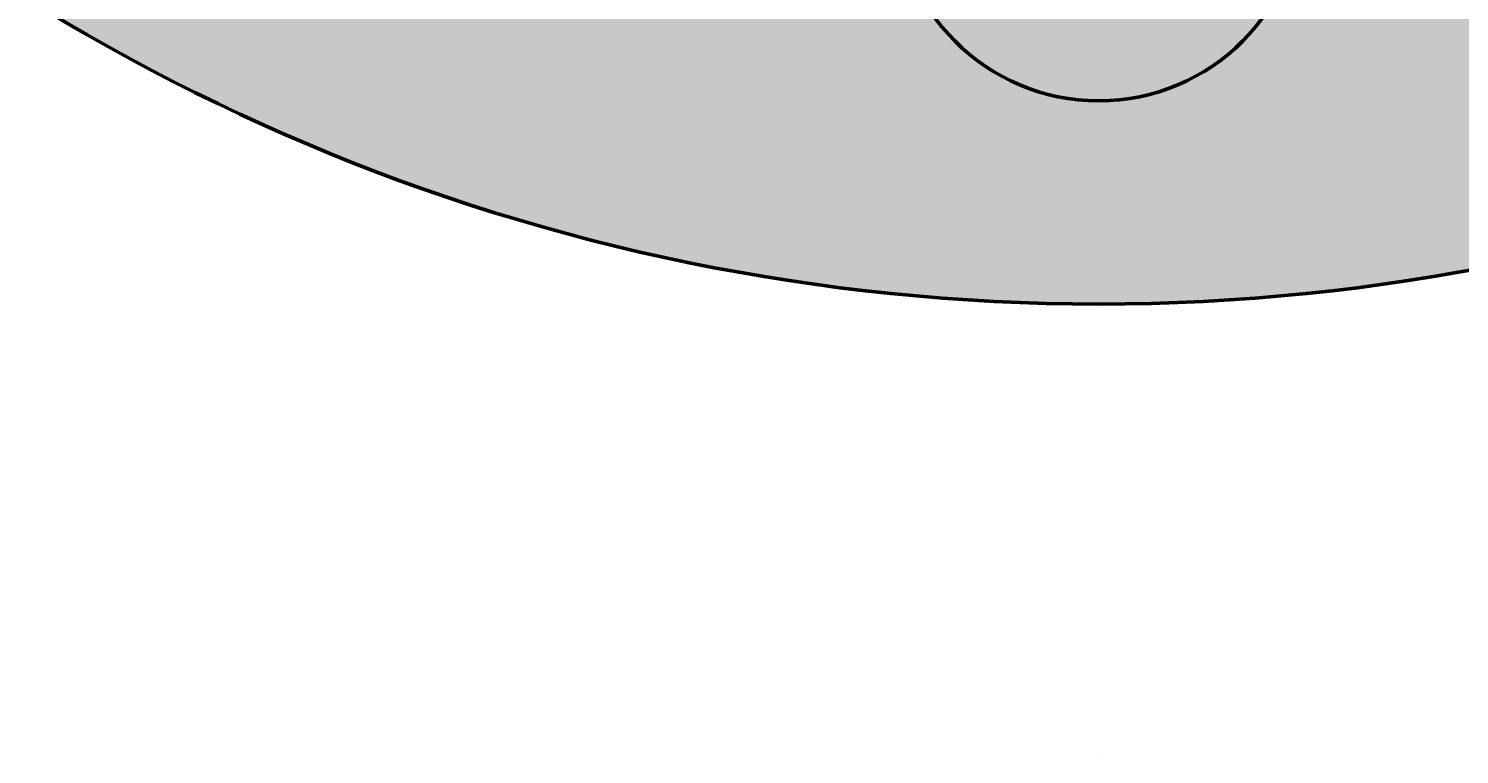
# Model space of a CAD drawing. Units: inches. Extents: x 139261 to 139415, y 52839 to 52963.
# Tile 7 of 20: x 139314 to 139349, y 52839 to 52857. Entities that reach past the tile are written whole.
import ezdxf

# ---------------------------------------------------------------- set-up
doc = ezdxf.new("R2010")
doc.units = ezdxf.units.IN
doc.header["$MEASUREMENT"] = 0
for name, color, linetype, lineweight in [('M-CONS', 9, 'Continuous', 13), ('M-DIMS', 2, 'Continuous', 25), ('M-HATC', 8, 'Continuous', 18), ('M-OUTL', 7, 'Continuous', 50)]:
    doc.layers.add(name, color=color, linetype=linetype, lineweight=lineweight)
doc.styles.get("Standard").update_dxf_attribs({"font": 'arial.ttf'})
doc.dimstyles.get("Standard").update_dxf_attribs({"dimtxt": 0.18, "dimasz": 0.18, "dimexe": 0.18, "dimexo": 0.0625, "dimgap": 0.09, "dimtad": 0, "dimtih": 1, "dimtoh": 1, "dimdec": 4, "dimzin": 0, "dimdsep": 46, "dimtxsty": 'Standard', "dimcen": 0.09, "dimadec": 0, "dimazin": 0, "dimtfac": 1, "dimtdec": 4, "dimtofl": 0, "dimtmove": 0, "dimatfit": 3, "dimfxl": 1, "dimtolj": 1, "dimtzin": 0, "dimarcsym": 0})

# ---------------------------------------------------------------- blocks, each defined once
blk = doc.blocks.new('*U1')
blk.add_circle((0, 0), 5)
blk = doc.blocks.new('*U2')
at = {"layer": 'M-OUTL', "color": 0, "linetype": 'ByBlock', "lineweight": -2, "transparency": 16777216, "rotation": 180}
blk.add_blockref('*U1', (139340.357, 52860.217), dxfattribs=at)
blk = doc.blocks.new('*D6')
at = {"layer": 'Defpoints', "color": 0, "transparency": 16777216}
for p in [(139332.153, 52949.54), (139348.561, 52850.895)]:
    blk.add_point(p, dxfattribs=at)
at = {"layer": 'M-DIMS', "color": 0, "lineweight": -2, "transparency": 16777216}
for p, q in [((139329.787, 52962.682), (139329.967, 52962.682)), ((139329.967, 52962.682), (139332.124, 52949.717)), ((139340.267, 52900.217), (139340.447, 52900.217)), ((139340.357, 52900.127), (139340.357, 52900.307))]:
    blk.add_line(p, q, dxfattribs=at)
at = {"layer": 'M-DIMS', "color": 0, "transparency": 16777216}
blk.add_solid([(139332.153, 52949.722), (139332.094, 52949.713), (139332.153, 52949.54)], dxfattribs=at)
at = {"layer": 'M-DIMS', "color": 0, "transparency": 16777216, "insert": (139329.086, 52962.682), "char_height": 0.18, "attachment_point": 5}
blk.add_mtext('\\A1;∅100.0000', dxfattribs=at)
blk = doc.blocks.new('*D10')
at = {"layer": 'Defpoints', "color": 0, "transparency": 16777216}
for p in [(139325.07, 52937.181), (139355.644, 52863.254)]:
    blk.add_point(p, dxfattribs=at)
at = {"layer": 'M-DIMS', "color": 0, "lineweight": -2, "transparency": 16777216}
for p, q in [((139340.267, 52900.217), (139340.447, 52900.217)), ((139340.357, 52900.127), (139340.357, 52900.307)), ((139364.816, 52841.075), (139355.712, 52863.087)), ((139364.996, 52841.075), (139364.816, 52841.075))]:
    blk.add_line(p, q, dxfattribs=at)
at = {"layer": 'M-DIMS', "color": 0, "transparency": 16777216}
blk.add_solid([(139355.74, 52863.099), (139355.685, 52863.076), (139355.644, 52863.254)], dxfattribs=at)
at = {"layer": 'M-DIMS', "color": 0, "transparency": 16777216, "insert": (139365.312, 52841.075), "char_height": 0.18, "attachment_point": 5}
blk.add_mtext('\\A1;∅80', dxfattribs=at)

msp = doc.modelspace()

# ---------------------------------------------------------------- hatches: boundary and pattern name
at = {"layer": 'M-HATC'}
h = msp.add_hatch(color=256, dxfattribs=at)
h.dxf.hatch_style = 1
h.paths.add_polyline_path([(139290.35689, 52900.21749, 1), (139390.35689, 52900.21749, 1)])
h.paths.add_polyline_path([(139335.36666, 52939.90499, -0.01563646), (139335.35689, 52940.21749, -1), (139345.35689, 52940.21749, -0.01563646), (139345.34711, 52939.90499, -0.13461315), (139364.89157, 52931.80941, -0.691035), (139373.64116, 52928.50176, -0.21521822), (139371.94881, 52924.75216, -0.13461315), (139380.04439, 52905.20771, -0.43265224), (139385.35689, 52900.21749, -0.43265224), (139380.04439, 52895.22726, -0.13461315), (139371.94881, 52875.68281, -0.21521822), (139373.64116, 52871.93321, -0.691035), (139364.89157, 52868.62556, -0.13461315), (139345.34711, 52860.52999, -0.01563646), (139345.35689, 52860.21749, -1), (139335.35689, 52860.21749, -0.01563646), (139335.36666, 52860.52999, -0.13461315), (139315.82221, 52868.62556, -0.691035), (139307.07262, 52871.93321, -0.21521822), (139308.76496, 52875.68281, -0.13461315), (139300.66939, 52895.22726, -0.43265224), (139295.35689, 52900.21749, -0.43265224), (139300.66939, 52905.20771, -0.13461315), (139308.76496, 52924.75216, -0.21521822), (139307.07262, 52928.50176, -0.691035), (139315.82221, 52931.80941, -0.13461315)], flags=16)
h.paths.add_polyline_path([(139365.35689, 52900.21749, -1), (139315.35689, 52900.21749, -1)], flags=0)
h.paths.add_polyline_path([(139323.71474, 52911.30978), (139356.99903, 52911.30978, -0.3027197), (139356.99903, 52889.12519), (139323.71474, 52889.12519, -0.3027197)], flags=0)
h.paths.add_polyline_path([(139364.89157, 52931.80941, 0.13461315), (139345.34711, 52939.90499, -0.93933644), (139335.36666, 52939.90499, 0.13461315), (139315.82221, 52931.80941, -0.18270763), (139317.07262, 52928.50176, -0.64579494), (139308.76496, 52924.75216, 0.13461315), (139300.66939, 52905.20771, -0.39601219), (139305.35689, 52900.21749, -0.39601219), (139300.66939, 52895.22726, 0.13461315), (139308.76496, 52875.68281, -0.64579494), (139317.07262, 52871.93321, -0.18270763), (139315.82221, 52868.62556, 0.13461315), (139335.36666, 52860.52999, -0.93933644), (139345.34711, 52860.52999, 0.13461315), (139364.89157, 52868.62556, -0.18270763), (139363.64116, 52871.93321, -0.64579494), (139371.94881, 52875.68281, 0.13461315), (139380.04439, 52895.22726, -0.39601219), (139375.35689, 52900.21749, -0.39601219), (139380.04439, 52905.20771, 0.13461315), (139371.94881, 52924.75216, -0.64579494), (139363.64116, 52928.50176, -0.18270763)], flags=0)
h = msp.add_hatch(color=256, dxfattribs=at)
h.dxf.hatch_style = 1
h.set_gradient(color1=(205, 105, 40), tint=1)
h.paths.add_polyline_path([(139335.35689, 52940.21749, 1), (139345.35689, 52940.21749, 1)])
h.paths.add_polyline_path([(139307.07262, 52928.50176, 1), (139317.07262, 52928.50176, 1)])
h.paths.add_polyline_path([(139295.35689, 52900.21749, 1), (139305.35689, 52900.21749, 1)])
h.paths.add_polyline_path([(139307.07262, 52871.93321, 1), (139317.07262, 52871.93321, 1)])
h.paths.add_polyline_path([(139345.35689, 52860.21749, 1), (139335.35689, 52860.21749, 1)])
h.paths.add_polyline_path([(139363.64116, 52871.93321, 1), (139373.64116, 52871.93321, 1)])
h.paths.add_polyline_path([(139375.35689, 52900.21749, 1), (139385.35689, 52900.21749, 1)])
h.paths.add_polyline_path([(139363.64116, 52928.50176, 1), (139373.64116, 52928.50176, 1)])

# ---------------------------------------------------------------- linework, layer by layer
at = {"layer": 'M-CONS'}
msp.add_line((139340.35689, 52839.13973), (139340.35689, 52839.13973), dxfattribs=at)
at = {"layer": 'M-OUTL'}
msp.add_circle((139340.35689, 52900.21749), 50, dxfattribs=at)

# ---------------------------------------------------------------- block references
msp.add_blockref('*U2', (0, 0), dxfattribs=at)

# ---------------------------------------------------------------- dimensions: what is measured, and where the dimension line sits
at = {"layer": 'M-DIMS'}
for p1, p2, override, picture, middle in [((139348.56051, 52850.89507), (139332.15326, 52949.5399), {"dimclrd": 0, "dimclre": 0, "dimclrt": 0}, '*D6', (139329.08622, 52962.68242)), ((139325.07023, 52937.18123), (139355.64354, 52863.25374), {"dimdec": 0, "dimlfac": 1, "dimrnd": 0, "dimzin": 0, "dimdsep": 46, "dimlunit": 2}, '*D10', (139365.31206, 52841.0755))]:
    dim = msp.add_diameter_dim_2p(p1=p1, p2=p2, dimstyle='Standard', override=override, dxfattribs=at)
    dim.commit()
    dim.dimension.update_dxf_attribs({"geometry": picture, "text_midpoint": middle, "dimtype": 163})

doc.saveas('drawing.dxf')
